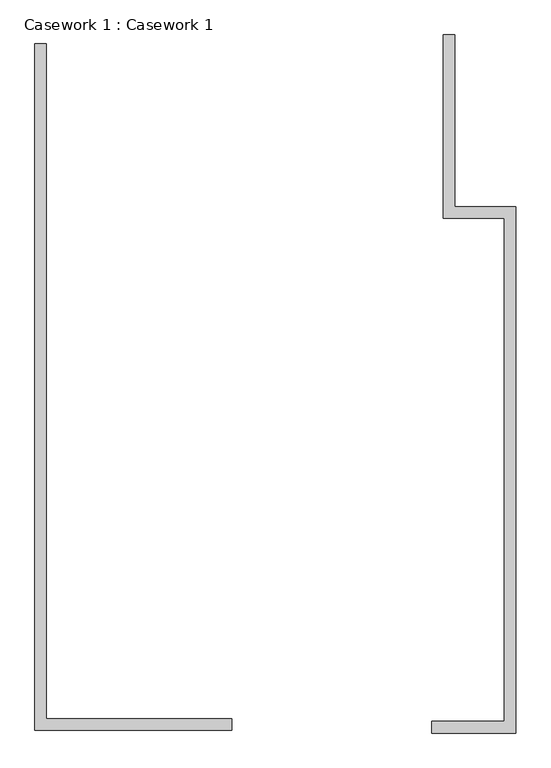
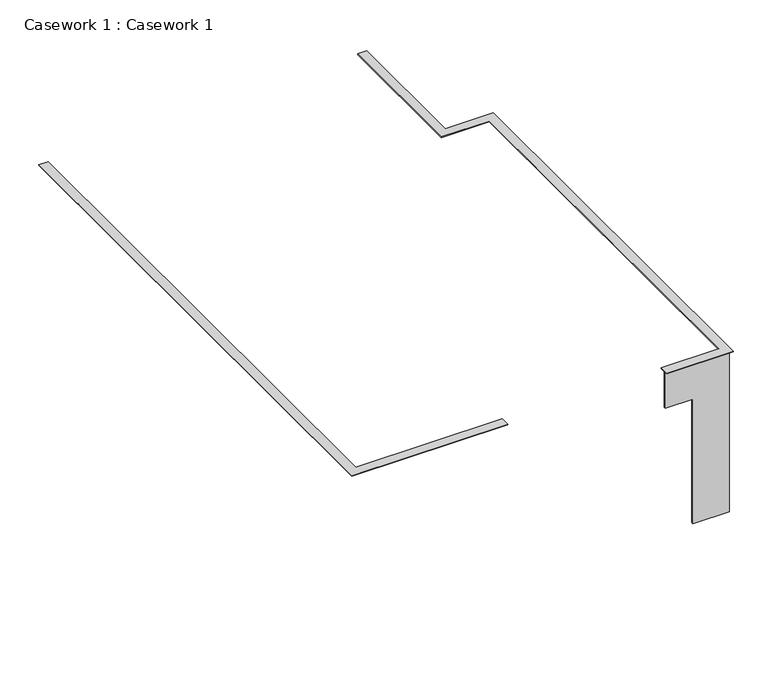
"""IFC4 building model written with IfcOpenShell, lengths in millimetres: furniture geometry, Casework 1 : Casework 1."""

from ifc_helpers import new_model, si_unit, frame, origin, place, context, project, spatial, polyline, outline, extrude, source, transform, mapped, element, save


def casework_1_casework_1_d55a6497(model_context):
    return source(origin(), model_context, "Body", "SweptSolid", [
        extrude(outline(polyline([(-8960.4564803, 5077.4735), (-8660.4564803, 5077.4735), (-8660.4564803, -12397.5265), (-3860.4564803, -12397.5265), (-3860.4564803, -12697.5265), (-8960.4564803, -12697.5265), (-8960.4564803, 5077.4735)])), frame((0.0, 0.0, 5550.0), z_axis=(0.0, 0.0, 1.0), x_axis=(1.0, 0.0, 0.0)), (0.0, 0.0, 1.0), 25.0),
        extrude(outline(polyline([(1314.5435197, -12772.5265), (1314.5435197, -12472.5265), (3189.5435197, -12472.5265), (3189.5435197, 552.4735), (1614.5435197, 552.4735), (1614.5435197, 5302.4735), (1914.5435197, 5302.4735), (1914.5435197, 852.4735), (3489.5435197, 852.4735), (3489.5435197, -12772.5265), (1314.5435197, -12772.5265)])), frame((0.0, 0.0, 5550.0), z_axis=(0.0, 0.0, 1.0), x_axis=(1.0, 0.0, 0.0)), (0.0, 0.0, 1.0), 25.0),
        extrude(outline(polyline([(5550.0, 3414.5435197), (5550.0, 1314.5435197), (4310.0, 1314.5435197), (4310.0, 2214.5435197), (0.0, 2214.5435197), (0.0, 3414.5435197), (5550.0, 3414.5435197)])), frame((0.0, -12697.5265, 0.0), z_axis=(0.0, 1.0, 0.0), x_axis=(0.0, 0.0, 1.0)), (0.0, 0.0, 1.0), 75.0),
    ])


if __name__ == "__main__":
    model = new_model("IFC4")
    model_context = context("Model", 3, world=origin())
    ifc_project = project(units=[si_unit("LENGTHUNIT", "METRE", prefix="MILLI")], contexts=[model_context])
    site = spatial("IfcSite", under=ifc_project)
    building = spatial("IfcBuilding", under=site)
    placement = place(None, origin())
    casework_1_casework_1_shape = casework_1_casework_1_d55a6497(model_context)
    element("IfcFurniture", 1, ObjectType="Casework 1 : Casework 1", at=placement, inside=building, context=model_context, shape_type="MappedRepresentation", body=[
        mapped(casework_1_casework_1_shape, transform((0.0, 0.0, 0.0), x_axis=(1.0, 0.0, 0.0), y_axis=(0.0, 1.0, 0.0), z_axis=(0.0, 0.0, 1.0))),
    ])
    save(model, "model.ifc")
